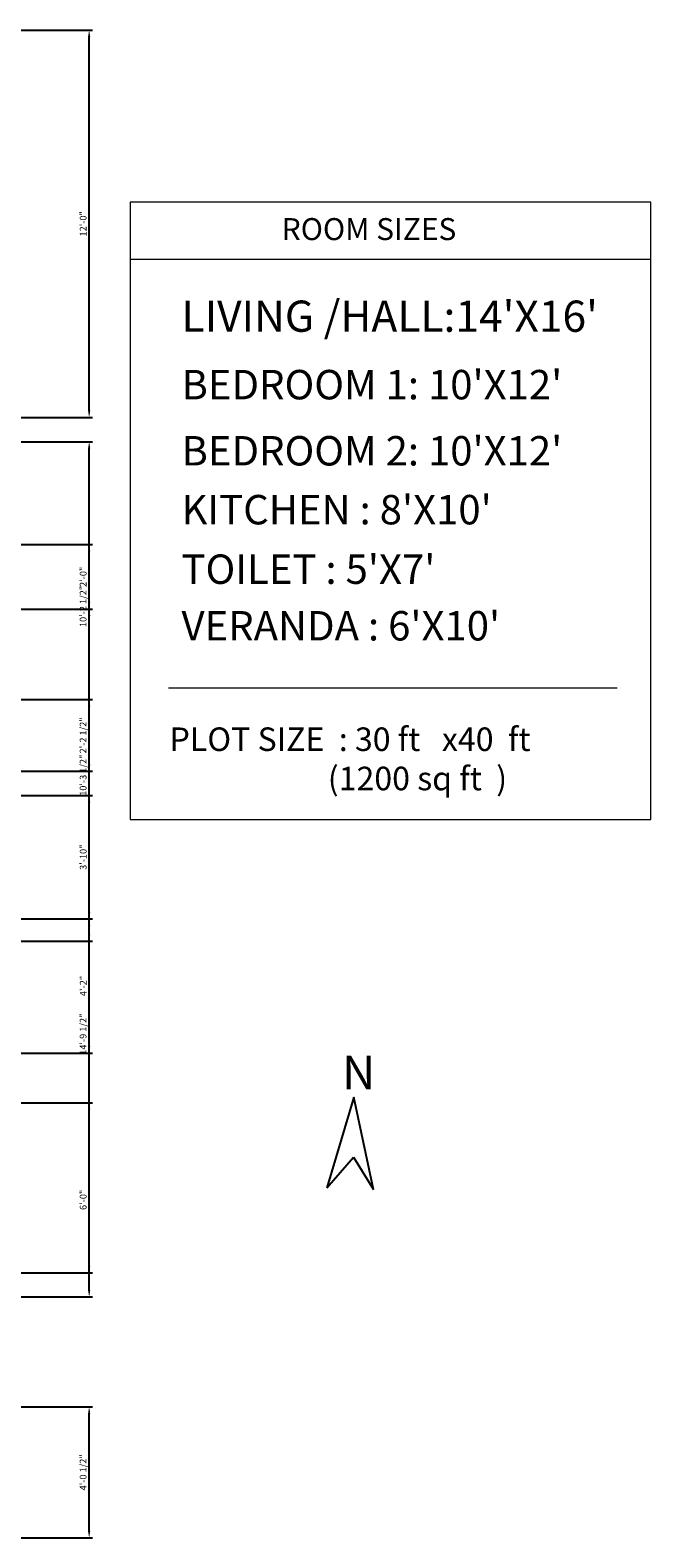
# Model space of a CAD drawing. Units: inches. Extents: x 655 to 1311, y 444 to 1096.
# Tile 4 of 4: x 1080 to 1311, y 478 to 1039. Entities that reach past the tile are written whole.
import ezdxf

# ---------------------------------------------------------------- set-up
doc = ezdxf.new("R2010")
doc.units = ezdxf.units.IN
for name, color, linetype, lineweight in [('A-ANNO-DIMS', 7, 'Continuous', 18), ('A-ANNO-SCHD', 7, 'Continuous', 18), ('A-ANNO-SYMB', 7, 'Continuous', 25), ('A-ANNO-TEXT', 7, 'Continuous', 18)]:
    doc.layers.add(name, color=color, linetype=linetype, lineweight=lineweight)
doc.styles.get("Standard").update_dxf_attribs({"font": 'arial.ttf'})
doc.dimstyles.new('ISO-25', dxfattribs={"dimtxt": 2.5, "dimasz": 2.5, "dimexe": 1.25, "dimexo": 0.625, "dimtad": 1, "dimdec": 0, "dimlunit": 3, "dimtxsty": 'Standard', "dimcen": 2.5, "dimadec": 0, "dimazin": 0, "dimtfac": 1, "dimtdec": 0, "dimtmove": 0, "dimatfit": 3, "dimfxl": 1, "dimarcsym": 0})

# ---------------------------------------------------------------- blocks, each defined once
blk = doc.blocks.new('*D23')
at = {"layer": 'A-ANNO-DIMS', "color": 0, "lineweight": -2, "transparency": 16777216}
for p, q in [((1060.96, 1038.75), (1102.98, 1038.75)), ((1101.73, 897.25), (1101.73, 1036.25)), ((1060.96, 894.75), (1102.98, 894.75))]:
    blk.add_line(p, q, dxfattribs=at)
at = {"layer": 'A-ANNO-DIMS', "color": 0, "transparency": 16777216}
for points in [[(1101.32, 1036.25), (1102.15, 1036.25), (1101.73, 1038.75)], [(1101.32, 897.25), (1102.15, 897.25), (1101.73, 894.75)]]:
    blk.add_solid(points, dxfattribs=at)
at = {"layer": 'Defpoints', "color": 0, "transparency": 16777216}
for p in [(1060.33, 1038.75), (1101.73, 1038.75), (1060.33, 894.75)]:
    blk.add_point(p, dxfattribs=at)
at = {"layer": 'A-ANNO-DIMS', "color": 0, "transparency": 16777216, "insert": (1099.83, 966.75), "char_height": 2.5, "attachment_point": 5, "rotation": 90}
blk.add_mtext('12\'-0"', dxfattribs=at)
blk = doc.blocks.new('*D25')
at = {"layer": 'A-ANNO-DIMS', "color": 0, "lineweight": -2, "transparency": 16777216}
for p, q in [((1060.96, 885.75), (1102.98, 885.75)), ((1101.73, 765.73), (1101.73, 883.25)), ((1060.96, 763.23), (1102.98, 763.23))]:
    blk.add_line(p, q, dxfattribs=at)
at = {"layer": 'A-ANNO-DIMS', "color": 0, "transparency": 16777216}
for points in [[(1101.32, 883.25), (1102.15, 883.25), (1101.73, 885.75)], [(1101.32, 765.73), (1102.15, 765.73), (1101.73, 763.23)]]:
    blk.add_solid(points, dxfattribs=at)
at = {"layer": 'Defpoints', "color": 0, "transparency": 16777216}
for p in [(1060.33, 885.75), (1101.73, 885.75), (1060.33, 763.23)]:
    blk.add_point(p, dxfattribs=at)
at = {"layer": 'A-ANNO-DIMS', "color": 0, "transparency": 16777216, "insert": (1099.81, 824.49), "char_height": 2.5, "attachment_point": 5, "rotation": 90}
blk.add_mtext('10\'-2 1/2"', dxfattribs=at)
blk = doc.blocks.new('*D26')
at = {"layer": 'A-ANNO-DIMS', "color": 0, "lineweight": -2, "transparency": 16777216}
for p, q in [((1069.96, 847.5), (1102.98, 847.5)), ((1101.73, 826), (1101.73, 845)), ((1069.96, 823.5), (1102.98, 823.5))]:
    blk.add_line(p, q, dxfattribs=at)
at = {"layer": 'A-ANNO-DIMS', "color": 0, "transparency": 16777216}
for points in [[(1101.32, 845), (1102.15, 845), (1101.73, 847.5)], [(1101.32, 826), (1102.15, 826), (1101.73, 823.5)]]:
    blk.add_solid(points, dxfattribs=at)
at = {"layer": 'Defpoints', "color": 0, "transparency": 16777216}
for p in [(1069.33, 847.5), (1101.73, 847.5), (1069.33, 823.5)]:
    blk.add_point(p, dxfattribs=at)
at = {"layer": 'A-ANNO-DIMS', "color": 0, "transparency": 16777216, "insert": (1099.83, 835.5), "char_height": 2.5, "attachment_point": 5, "rotation": 90}
blk.add_mtext('2\'-0"', dxfattribs=at)
blk = doc.blocks.new('*D27')
at = {"layer": 'A-ANNO-DIMS', "color": 0, "lineweight": -2, "transparency": 16777216}
for p, q in [((1069.96, 823.5), (1102.98, 823.5)), ((1101.73, 702.49), (1101.73, 821)), ((1069.96, 699.99), (1102.98, 699.99))]:
    blk.add_line(p, q, dxfattribs=at)
at = {"layer": 'A-ANNO-DIMS', "color": 0, "transparency": 16777216}
for points in [[(1101.32, 821), (1102.15, 821), (1101.73, 823.5)], [(1101.32, 702.49), (1102.15, 702.49), (1101.73, 699.99)]]:
    blk.add_solid(points, dxfattribs=at)
at = {"layer": 'Defpoints', "color": 0, "transparency": 16777216}
for p in [(1069.33, 823.5), (1101.73, 823.5), (1069.33, 699.99)]:
    blk.add_point(p, dxfattribs=at)
at = {"layer": 'A-ANNO-DIMS', "color": 0, "transparency": 16777216, "insert": (1099.81, 761.75), "char_height": 2.5, "attachment_point": 5, "rotation": 90}
blk.add_mtext('10\'-3 1/2"', dxfattribs=at)
blk = doc.blocks.new('*D28')
at = {"layer": 'A-ANNO-DIMS', "color": 0, "lineweight": -2, "transparency": 16777216}
for p, q in [((1069.96, 639.99), (1102.98, 639.99)), ((1101.73, 570.25), (1101.73, 637.49)), ((1069.96, 567.75), (1102.98, 567.75))]:
    blk.add_line(p, q, dxfattribs=at)
at = {"layer": 'A-ANNO-DIMS', "color": 0, "transparency": 16777216}
for points in [[(1101.32, 637.49), (1102.15, 637.49), (1101.73, 639.99)], [(1101.32, 570.25), (1102.15, 570.25), (1101.73, 567.75)]]:
    blk.add_solid(points, dxfattribs=at)
at = {"layer": 'Defpoints', "color": 0, "transparency": 16777216}
for p in [(1069.33, 639.99), (1101.73, 639.99), (1069.33, 567.75)]:
    blk.add_point(p, dxfattribs=at)
at = {"layer": 'A-ANNO-DIMS', "color": 0, "transparency": 16777216, "insert": (1099.83, 603.87), "char_height": 2.5, "attachment_point": 5, "rotation": 90}
blk.add_mtext('6\'-0"', dxfattribs=at)
blk = doc.blocks.new('*D32')
at = {"layer": 'A-ANNO-DIMS', "color": 0, "lineweight": -2, "transparency": 16777216}
for p, q in [((1055.1, 789.89), (1102.98, 789.89)), ((1101.73, 765.69), (1101.73, 787.39)), ((1055.1, 763.19), (1102.98, 763.19))]:
    blk.add_line(p, q, dxfattribs=at)
at = {"layer": 'A-ANNO-DIMS', "color": 0, "transparency": 16777216}
for points in [[(1101.32, 787.39), (1102.15, 787.39), (1101.73, 789.89)], [(1101.32, 765.69), (1102.15, 765.69), (1101.73, 763.19)]]:
    blk.add_solid(points, dxfattribs=at)
at = {"layer": 'Defpoints', "color": 0, "transparency": 16777216}
for p in [(1054.47, 789.89), (1101.73, 789.89), (1054.47, 763.19)]:
    blk.add_point(p, dxfattribs=at)
at = {"layer": 'A-ANNO-DIMS', "color": 0, "transparency": 16777216, "insert": (1099.81, 776.54), "char_height": 2.5, "attachment_point": 5, "rotation": 90}
blk.add_mtext('2\'-2 1/2"', dxfattribs=at)
blk = doc.blocks.new('*D36')
at = {"layer": 'A-ANNO-DIMS', "color": 0, "lineweight": -2, "transparency": 16777216}
for p, q in [((1060.96, 754.19), (1102.98, 754.19)), ((1101.73, 579.25), (1101.73, 751.69)), ((1060.96, 576.75), (1102.98, 576.75))]:
    blk.add_line(p, q, dxfattribs=at)
at = {"layer": 'A-ANNO-DIMS', "color": 0, "transparency": 16777216}
for points in [[(1101.32, 751.69), (1102.15, 751.69), (1101.73, 754.19)], [(1101.32, 579.25), (1102.15, 579.25), (1101.73, 576.75)]]:
    blk.add_solid(points, dxfattribs=at)
at = {"layer": 'Defpoints', "color": 0, "transparency": 16777216}
for p in [(1060.33, 754.19), (1101.73, 754.19), (1060.33, 576.75)]:
    blk.add_point(p, dxfattribs=at)
at = {"layer": 'A-ANNO-DIMS', "color": 0, "transparency": 16777216, "insert": (1099.81, 665.47), "char_height": 2.5, "attachment_point": 5, "rotation": 90}
blk.add_mtext('14\'-9 1/2"', dxfattribs=at)
blk = doc.blocks.new('*D42')
at = {"layer": 'A-ANNO-DIMS', "color": 0, "lineweight": -2, "transparency": 16777216}
for p, q in [((1058.6, 708.34), (1102.98, 708.34)), ((1101.73, 660.93), (1101.73, 705.84)), ((1058.6, 658.43), (1102.98, 658.43))]:
    blk.add_line(p, q, dxfattribs=at)
at = {"layer": 'A-ANNO-DIMS', "color": 0, "transparency": 16777216}
for points in [[(1101.32, 705.84), (1102.15, 705.84), (1101.73, 708.34)], [(1101.32, 660.93), (1102.15, 660.93), (1101.73, 658.43)]]:
    blk.add_solid(points, dxfattribs=at)
at = {"layer": 'Defpoints', "color": 0, "transparency": 16777216}
for p in [(1057.97, 708.34), (1101.73, 708.34), (1057.97, 658.43)]:
    blk.add_point(p, dxfattribs=at)
at = {"layer": 'A-ANNO-DIMS', "color": 0, "transparency": 16777216, "insert": (1099.85, 683.38), "char_height": 2.5, "attachment_point": 5, "rotation": 90}
blk.add_mtext('4\'-2"', dxfattribs=at)
blk = doc.blocks.new('*D43')
at = {"layer": 'A-ANNO-DIMS', "color": 0, "lineweight": -2, "transparency": 16777216}
for p, q in [((1060.96, 754.19), (1102.98, 754.19)), ((1101.73, 710.84), (1101.73, 751.69)), ((1058.6, 708.34), (1102.98, 708.34))]:
    blk.add_line(p, q, dxfattribs=at)
at = {"layer": 'A-ANNO-DIMS', "color": 0, "transparency": 16777216}
for points in [[(1101.32, 751.69), (1102.15, 751.69), (1101.73, 754.19)], [(1101.32, 710.84), (1102.15, 710.84), (1101.73, 708.34)]]:
    blk.add_solid(points, dxfattribs=at)
at = {"layer": 'Defpoints', "color": 0, "transparency": 16777216}
for p in [(1060.33, 754.19), (1101.73, 754.19), (1057.97, 708.34)]:
    blk.add_point(p, dxfattribs=at)
at = {"layer": 'A-ANNO-DIMS', "color": 0, "transparency": 16777216, "insert": (1099.83, 731.26), "char_height": 2.5, "attachment_point": 5, "rotation": 90}
blk.add_mtext('3\'-10"', dxfattribs=at)
blk = doc.blocks.new('*D52')
at = {"layer": 'A-ANNO-DIMS', "color": 0, "lineweight": -2, "transparency": 16777216}
for p, q in [((1069.96, 526.9), (1102.98, 526.9)), ((1101.73, 480.7), (1101.73, 524.4)), ((1069.96, 478.2), (1102.98, 478.2))]:
    blk.add_line(p, q, dxfattribs=at)
at = {"layer": 'A-ANNO-DIMS', "color": 0, "transparency": 16777216}
for points in [[(1101.32, 524.4), (1102.15, 524.4), (1101.73, 526.9)], [(1101.32, 480.7), (1102.15, 480.7), (1101.73, 478.2)]]:
    blk.add_solid(points, dxfattribs=at)
at = {"layer": 'Defpoints', "color": 0, "transparency": 16777216}
for p in [(1069.33, 526.9), (1101.73, 526.9), (1069.33, 478.2)]:
    blk.add_point(p, dxfattribs=at)
at = {"layer": 'A-ANNO-DIMS', "color": 0, "transparency": 16777216, "insert": (1099.81, 502.55), "char_height": 2.5, "attachment_point": 5, "rotation": 90}
blk.add_mtext('4\'-0 1/2"', dxfattribs=at)

msp = doc.modelspace()

# ---------------------------------------------------------------- linework, layer by layer
at = {"layer": 'A-ANNO-SCHD'}
for p, q in [((1310.64, 974.85), (1117.04, 974.85)), ((1117.04, 974.85), (1117.04, 745.3)), ((1310.64, 745.3), (1310.64, 974.85)), ((1310.64, 953.49), (1117.04, 953.49)), ((1131.2, 794.19), (1298.14, 794.19)), ((1117.04, 745.3), (1310.64, 745.3))]:
    msp.add_line(p, q, dxfattribs=at)
at = {"layer": 'A-ANNO-SYMB'}
for p, q in [((1200.2, 642.02), (1190.14, 608.29)), ((1207.46, 607.7), (1200.2, 642.02)), ((1190.14, 608.29), (1199.99, 619.78)), ((1199.99, 619.78), (1207.46, 607.7))]:
    msp.add_line(p, q, dxfattribs=at)

# ---------------------------------------------------------------- texts
at = {"layer": 'A-ANNO-SYMB', "insert": (1195.82, 657.44), "char_height": 12.5, "attachment_point": 1}
msp.add_mtext_dynamic_manual_height_columns('N', width=124.1281, gutter_width=62.5, heights=[0], dxfattribs=at)
at = {"layer": 'A-ANNO-TEXT', "attachment_point": 1}
for s, width, gutter_width, insert, char_height in [('ROOM SIZES', 109.8506, 40.81, (1173.35, 968.87), 8.162), ("LIVING /HALL:14'X16'", 379.3713, 58.04, (1136.08, 938.21), 11.6074), ("BEDROOM 1: 10'X12'", 301.8384, 54.67, (1136.08, 912.42), 10.9331), ("BEDROOM 2: 10'X12'", 301.8384, 54.67, (1136.08, 887.83), 10.9331), ("KITCHEN : 8'X10'", 301.8384, 54.67, (1136.08, 865.94), 10.9331), ("TOILET : 5'X7'", 301.8384, 54.67, (1136.08, 843.81), 10.9331), ("VERANDA : 6'X10'", 301.8384, 54.67, (1136.08, 822.77), 10.9331), ('PLOT SIZE  : 30 ft   x40  ft\\P                      (1200 sq ft  )', 162.0052, 43.78, (1131.63, 779.5), 8.7558)]:
    msp.add_mtext_dynamic_manual_height_columns(s, width=width, gutter_width=gutter_width, heights=[0], dxfattribs=dict(at, insert=insert, char_height=char_height))

# ---------------------------------------------------------------- dimensions: what is measured, and where the dimension line sits
at = {"layer": 'A-ANNO-DIMS'}
for base, p1, p2, picture, middle in [((1101.73, 1038.75), (1060.33, 894.75), (1060.33, 1038.75), '*D23', (1099.83, 966.75)), ((1101.73, 885.75), (1060.33, 763.23), (1060.33, 885.75), '*D25', (1099.81, 824.49)), ((1101.73, 847.5), (1069.33, 823.5), (1069.33, 847.5), '*D26', (1099.83, 835.5)), ((1101.73, 823.5), (1069.33, 699.99), (1069.33, 823.5), '*D27', (1099.81, 761.75)), ((1101.73, 789.89), (1054.47, 763.19), (1054.47, 789.89), '*D32', (1099.81, 776.54)), ((1101.7326, 754.1916), (1057.971, 708.3354), (1060.3326, 754.1916), '*D43', (1099.8303, 731.2635)), ((1101.73, 754.19), (1060.33, 576.75), (1060.33, 754.19), '*D36', (1099.81, 665.47)), ((1101.73, 708.34), (1057.97, 658.43), (1057.97, 708.34), '*D42', (1099.85, 683.38)), ((1101.73, 639.99), (1069.33, 567.75), (1069.33, 639.99), '*D28', (1099.83, 603.87)), ((1101.73, 526.9), (1069.33, 478.2), (1069.33, 526.9), '*D52', (1099.81, 502.55))]:
    dim = msp.add_linear_dim(base=base, p1=p1, p2=p2, angle=90, dimstyle='ISO-25', override={"dimdec": 1, "dimlfac": 1, "dimrnd": 0, "dimzin": 1, "dimdsep": 46, "dimlunit": 4, "dimfrac": 2}, dxfattribs=at)
    dim.commit()
    dim.dimension.update_dxf_attribs({"geometry": picture, "text_midpoint": middle})

doc.saveas('drawing.dxf')
